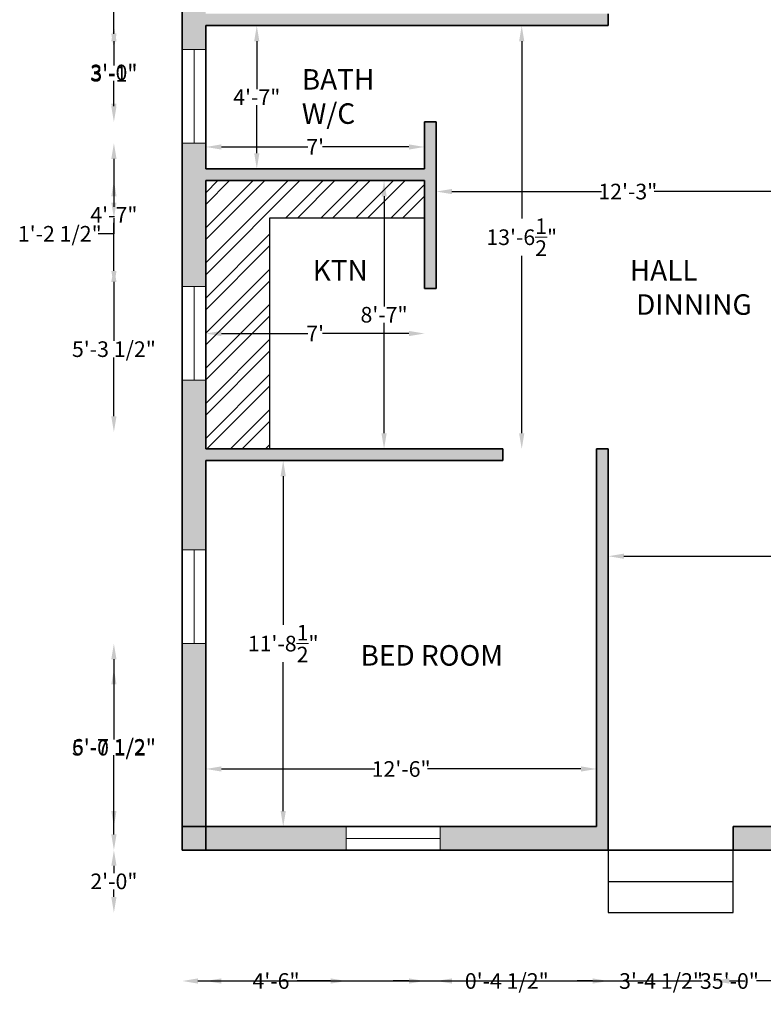
# Model space of a CAD drawing. Units: inches. Extents: x 759 to 1283, y 452 to 1038.
# Tile 1 of 3: x 759 to 1044, y 452 to 830. Entities that reach past the tile are written whole.
import ezdxf

# ---------------------------------------------------------------- set-up
doc = ezdxf.new("R2010")
doc.units = ezdxf.units.IN
for name, color, linetype, lineweight in [('A-AREA-IDEN', 1, 'Continuous', 25), ('A-COLS', 7, 'Continuous', 35), ('A-COLS-PATT', 7, 'Continuous', 13), ('A-FLOR-FIXT', 8, 'Continuous', 25), ('A-FLOR-FIXT-PATT', 7, 'Continuous', 13), ('DIM', 2, 'Continuous', 18), ('STAIR', 7, 'Continuous', 25), ('WALL', 7, 'Continuous', 35), ('WINDOWS', 4, 'Continuous', 18)]:
    doc.layers.add(name, color=color, linetype=linetype, lineweight=lineweight)
doc.layers.add('A-WALL-PATT', color=67, linetype='Continuous', lineweight=13, true_color=0x727430)
doc.styles.get("Standard").update_dxf_attribs({"font": 'arial.ttf'})
doc.dimstyles.get("Standard").update_dxf_attribs({"dimtxt": 6, "dimasz": 6, "dimexe": 0.18, "dimexo": 0.0625, "dimgap": 0.09, "dimtad": 0, "dimtih": 1, "dimtoh": 1, "dimdec": 4, "dimzin": 0, "dimdsep": 46, "dimlunit": 4, "dimtxsty": 'Standard', "dimcen": 0.09, "dimse1": 1, "dimse2": 1, "dimadec": 0, "dimazin": 0, "dimtfac": 1, "dimtdec": 4, "dimtofl": 0, "dimtmove": 0, "dimatfit": 3, "dimfxl": 1, "dimtolj": 1, "dimtzin": 0, "dimarcsym": 0})

# ---------------------------------------------------------------- blocks, each defined once
blk = doc.blocks.new('*D5')
at = {"layer": 'Defpoints', "color": 0, "transparency": 16777216}
for p in [(914.47, 780.7), (830.47, 772.31), (914.47, 772.31)]:
    blk.add_point(p, dxfattribs=at)
at = {"layer": 'DIM', "color": 0, "lineweight": -2, "transparency": 16777216}
for p, q in [((836.47, 780.7), (869.64, 780.7)), ((908.47, 780.7), (875.29, 780.7))]:
    blk.add_line(p, q, dxfattribs=at)
at = {"layer": 'DIM', "color": 0, "transparency": 16777216}
for points in [[(836.47, 781.7), (836.47, 779.7), (830.47, 780.7)], [(908.47, 781.7), (908.47, 779.7), (914.47, 780.7)]]:
    blk.add_solid(points, dxfattribs=at)
at = {"layer": 'DIM', "color": 0, "transparency": 16777216, "insert": (872.47, 780.7), "char_height": 6, "attachment_point": 5}
blk.add_mtext("\\A1;7'", dxfattribs=at)
blk = doc.blocks.new('*D6')
at = {"layer": 'Defpoints', "color": 0, "transparency": 16777216}
for p in [(830.47, 827.31), (830.47, 772.31), (850.06, 772.31)]:
    blk.add_point(p, dxfattribs=at)
at = {"layer": 'DIM', "color": 0, "lineweight": -2, "transparency": 16777216}
for p, q in [((850.06, 821.31), (850.06, 802.9)), ((850.06, 778.31), (850.06, 796.72))]:
    blk.add_line(p, q, dxfattribs=at)
at = {"layer": 'DIM', "color": 0, "transparency": 16777216}
for points in [[(849.06, 821.31), (851.06, 821.31), (850.06, 827.31)], [(849.06, 778.31), (851.06, 778.31), (850.06, 772.31)]]:
    blk.add_solid(points, dxfattribs=at)
at = {"layer": 'DIM', "color": 0, "transparency": 16777216, "insert": (850.06, 799.81), "char_height": 6, "attachment_point": 5}
blk.add_mtext('\\A1;4\'-7"', dxfattribs=at)
blk = doc.blocks.new('*D7')
at = {"layer": 'Defpoints', "color": 0, "transparency": 16777216}
for p in [(830.47, 767.81), (914.47, 767.81), (914.47, 709.09)]:
    blk.add_point(p, dxfattribs=at)
at = {"layer": 'DIM', "color": 0, "lineweight": -2, "transparency": 16777216}
for p, q in [((836.47, 709.09), (869.64, 709.09)), ((908.47, 709.09), (875.29, 709.09))]:
    blk.add_line(p, q, dxfattribs=at)
at = {"layer": 'DIM', "color": 0, "transparency": 16777216}
for points in [[(836.47, 710.09), (836.47, 708.09), (830.47, 709.09)], [(908.47, 710.09), (908.47, 708.09), (914.47, 709.09)]]:
    blk.add_solid(points, dxfattribs=at)
at = {"layer": 'DIM', "color": 0, "transparency": 16777216, "insert": (872.47, 709.09), "char_height": 6, "attachment_point": 5}
blk.add_mtext("\\A1;7'", dxfattribs=at)
blk = doc.blocks.new('*D8')
at = {"layer": 'Defpoints', "color": 0, "transparency": 16777216}
for p in [(830.47, 767.81), (830.47, 664.81), (898.91, 664.81)]:
    blk.add_point(p, dxfattribs=at)
at = {"layer": 'DIM', "color": 0, "lineweight": -2, "transparency": 16777216}
for p, q in [((898.91, 761.81), (898.91, 719.46)), ((898.91, 670.81), (898.91, 713.15))]:
    blk.add_line(p, q, dxfattribs=at)
at = {"layer": 'DIM', "color": 0, "transparency": 16777216}
for points in [[(897.91, 761.81), (899.91, 761.81), (898.91, 767.81)], [(897.91, 670.81), (899.91, 670.81), (898.91, 664.81)]]:
    blk.add_solid(points, dxfattribs=at)
at = {"layer": 'DIM', "color": 0, "transparency": 16777216, "insert": (898.91, 716.31), "char_height": 6, "attachment_point": 5}
blk.add_mtext('\\A1;8\'-7"', dxfattribs=at)
blk = doc.blocks.new('*D9')
at = {"layer": 'Defpoints', "color": 0, "transparency": 16777216}
for p in [(980.47, 541.94), (830.47, 519.81), (980.47, 519.81)]:
    blk.add_point(p, dxfattribs=at)
at = {"layer": 'DIM', "color": 0, "lineweight": -2, "transparency": 16777216}
for p, q in [((836.47, 541.94), (895.35, 541.94)), ((974.47, 541.94), (915.58, 541.94))]:
    blk.add_line(p, q, dxfattribs=at)
at = {"layer": 'DIM', "color": 0, "transparency": 16777216}
for points in [[(836.47, 542.94), (836.47, 540.94), (830.47, 541.94)], [(974.47, 542.94), (974.47, 540.94), (980.47, 541.94)]]:
    blk.add_solid(points, dxfattribs=at)
at = {"layer": 'DIM', "color": 0, "transparency": 16777216, "insert": (905.47, 541.94), "char_height": 6, "attachment_point": 5}
blk.add_mtext('\\A1;12\'-6"', dxfattribs=at)
blk = doc.blocks.new('*D10')
at = {"layer": 'Defpoints', "color": 0, "transparency": 16777216}
for p in [(830.47, 660.31), (830.47, 519.81), (860.2, 519.81)]:
    blk.add_point(p, dxfattribs=at)
at = {"layer": 'DIM', "color": 0, "lineweight": -2, "transparency": 16777216}
for p, q in [((860.2, 654.31), (860.2, 597.22)), ((860.2, 525.81), (860.2, 582.89))]:
    blk.add_line(p, q, dxfattribs=at)
at = {"layer": 'DIM', "color": 0, "transparency": 16777216}
for points in [[(859.2, 654.31), (861.2, 654.31), (860.2, 660.31)], [(859.2, 525.81), (861.2, 525.81), (860.2, 519.81)]]:
    blk.add_solid(points, dxfattribs=at)
at = {"layer": 'DIM', "color": 0, "transparency": 16777216, "insert": (860.2, 590.06), "char_height": 6, "attachment_point": 5}
blk.add_mtext('\\A1;11\'-8{\\H1x;\\S1/2;}"', dxfattribs=at)
blk = doc.blocks.new('*D12')
at = {"layer": 'Defpoints', "color": 0, "transparency": 16777216}
for p in [(1232.47, 623.61), (984.97, 524.08), (1232.47, 524.08)]:
    blk.add_point(p, dxfattribs=at)
at = {"layer": 'DIM', "color": 0, "lineweight": -2, "transparency": 16777216}
for p, q in [((990.97, 623.61), (1096.08, 623.61)), ((1226.47, 623.61), (1121.35, 623.61))]:
    blk.add_line(p, q, dxfattribs=at)
at = {"layer": 'DIM', "color": 0, "transparency": 16777216}
for points in [[(990.97, 624.61), (990.97, 622.61), (984.97, 623.61)], [(1226.47, 624.61), (1226.47, 622.61), (1232.47, 623.61)]]:
    blk.add_solid(points, dxfattribs=at)
at = {"layer": 'DIM', "color": 0, "transparency": 16777216, "insert": (1108.72, 623.61), "char_height": 6, "attachment_point": 5}
blk.add_mtext('\\A1;20\'-7{\\H1x;\\S1/2;}"', dxfattribs=at)
blk = doc.blocks.new('*D15')
at = {"layer": 'Defpoints', "color": 0, "transparency": 16777216}
for p in [(1065.97, 763.58), (918.97, 756.35), (1065.97, 756.35)]:
    blk.add_point(p, dxfattribs=at)
at = {"layer": 'DIM', "color": 0, "lineweight": -2, "transparency": 16777216}
for p, q in [((924.97, 763.58), (982.35, 763.58)), ((1059.97, 763.58), (1002.58, 763.58))]:
    blk.add_line(p, q, dxfattribs=at)
at = {"layer": 'DIM', "color": 0, "transparency": 16777216}
for points in [[(924.97, 764.58), (924.97, 762.58), (918.97, 763.58)], [(1059.97, 764.58), (1059.97, 762.58), (1065.97, 763.58)]]:
    blk.add_solid(points, dxfattribs=at)
at = {"layer": 'DIM', "color": 0, "transparency": 16777216, "insert": (992.47, 763.58), "char_height": 6, "attachment_point": 5}
blk.add_mtext('\\A1;12\'-3"', dxfattribs=at)
blk = doc.blocks.new('*D16')
at = {"layer": 'Defpoints', "color": 0, "transparency": 16777216}
for p in [(930.7, 827.31), (930.7, 664.81), (951.75, 664.81)]:
    blk.add_point(p, dxfattribs=at)
at = {"layer": 'DIM', "color": 0, "lineweight": -2, "transparency": 16777216}
for p, q in [((951.75, 821.31), (951.75, 753.22)), ((951.75, 670.81), (951.75, 738.89))]:
    blk.add_line(p, q, dxfattribs=at)
at = {"layer": 'DIM', "color": 0, "transparency": 16777216}
for points in [[(950.75, 821.31), (952.75, 821.31), (951.75, 827.31)], [(950.75, 670.81), (952.75, 670.81), (951.75, 664.81)]]:
    blk.add_solid(points, dxfattribs=at)
at = {"layer": 'DIM', "color": 0, "transparency": 16777216, "insert": (951.75, 746.06), "char_height": 6, "attachment_point": 5}
blk.add_mtext('\\A1;13\'-6{\\H1x;\\S1/2;}"', dxfattribs=at)
blk = doc.blocks.new('WIN-36IN')
for p, q in [((0, 0), (0, 9)), ((0, 9), (36, 9)), ((36, 9), (36, 0)), ((0, 4.5), (36, 4.5)), ((36, 0), (0, 0))]:
    blk.add_line(p, q)
blk = doc.blocks.new('COL-9X9IN')
for p, q in [((0, 0), (0, 9)), ((0, 9), (9, 9)), ((9, 9), (9, 0)), ((9, 0), (0, 0))]:
    blk.add_line(p, q)
blk = doc.blocks.new('*D23')
at = {"layer": 'Defpoints', "color": 0, "transparency": 16777216}
for p in [(821.47, 510.81), (1241.47, 510.81), (1241.47, 460.56)]:
    blk.add_point(p, dxfattribs=at)
at = {"layer": 'DIM', "color": 0, "lineweight": -2, "transparency": 16777216}
for p, q in [((827.47, 460.56), (1021.07, 460.56)), ((1235.47, 460.56), (1041.86, 460.56))]:
    blk.add_line(p, q, dxfattribs=at)
at = {"layer": 'DIM', "color": 0, "transparency": 16777216}
for points in [[(827.47, 461.56), (827.47, 459.56), (821.47, 460.56)], [(1235.47, 461.56), (1235.47, 459.56), (1241.47, 460.56)]]:
    blk.add_solid(points, dxfattribs=at)
at = {"layer": 'DIM', "color": 0, "transparency": 16777216, "insert": (1031.47, 460.56), "char_height": 6, "attachment_point": 5}
blk.add_mtext('\\A1;35\'-0"', dxfattribs=at)
blk = doc.blocks.new('*D24')
at = {"layer": 'Defpoints', "color": 0, "transparency": 16777216}
for p in [(1070.47, 1002.81), (1267.72, 1002.81), (1032.97, 486.81)]:
    blk.add_point(p, dxfattribs=at)
at = {"layer": 'DIM', "color": 0, "lineweight": -2, "transparency": 16777216}
for p, q in [((1267.72, 996.81), (1267.72, 747.96)), ((1267.72, 492.81), (1267.72, 741.65))]:
    blk.add_line(p, q, dxfattribs=at)
at = {"layer": 'DIM', "color": 0, "transparency": 16777216}
for points in [[(1266.72, 996.81), (1268.72, 996.81), (1267.72, 1002.81)], [(1266.72, 492.81), (1268.72, 492.81), (1267.72, 486.81)]]:
    blk.add_solid(points, dxfattribs=at)
at = {"layer": 'DIM', "color": 0, "transparency": 16777216, "insert": (1267.72, 744.81), "char_height": 6, "attachment_point": 5}
blk.add_mtext('\\A1;43\'-0"', dxfattribs=at)
blk = doc.blocks.new('*D27')
at = {"layer": 'Defpoints', "color": 0, "transparency": 16777216}
for p in [(1032.97, 1029.06), (984.97, 510.81), (1032.97, 510.81)]:
    blk.add_point(p, dxfattribs=at)
at = {"layer": 'DIM', "color": 0, "lineweight": -2, "transparency": 16777216}
for p, q in [((990.97, 1029.06), (1000.78, 1029.06)), ((1026.97, 1029.06), (1017.15, 1029.06))]:
    blk.add_line(p, q, dxfattribs=at)
at = {"layer": 'DIM', "color": 0, "transparency": 16777216}
for points in [[(990.97, 1030.06), (990.97, 1028.06), (984.97, 1029.06)], [(1026.97, 1030.06), (1026.97, 1028.06), (1032.97, 1029.06)]]:
    blk.add_solid(points, dxfattribs=at)
at = {"layer": 'DIM', "color": 0, "transparency": 16777216, "insert": (1008.97, 1029.06), "char_height": 6, "attachment_point": 5}
blk.add_mtext('\\A1;4\'-0"', dxfattribs=at)
blk = doc.blocks.new('*D28')
at = {"layer": 'Defpoints', "color": 0, "transparency": 16777216}
for p in [(795.22, 510.81), (984.97, 510.81), (984.97, 486.81)]:
    blk.add_point(p, dxfattribs=at)
at = {"layer": 'DIM', "color": 0, "lineweight": -2, "transparency": 16777216}
for p, q in [((795.22, 504.81), (795.22, 501.96)), ((795.22, 492.81), (795.22, 495.65))]:
    blk.add_line(p, q, dxfattribs=at)
at = {"layer": 'DIM', "color": 0, "transparency": 16777216}
for points in [[(794.22, 504.81), (796.22, 504.81), (795.22, 510.81)], [(794.22, 492.81), (796.22, 492.81), (795.22, 486.81)]]:
    blk.add_solid(points, dxfattribs=at)
at = {"layer": 'DIM', "color": 0, "transparency": 16777216, "insert": (795.22, 498.81), "char_height": 6, "attachment_point": 5}
blk.add_mtext('\\A1;2\'-0"', dxfattribs=at)
blk = doc.blocks.new('*D29')
at = {"layer": 'Defpoints', "color": 0, "transparency": 16777216}
for p in [(830.47, 981.81), (884.41, 981.81), (884.41, 460.56)]:
    blk.add_point(p, dxfattribs=at)
at = {"layer": 'DIM', "color": 0, "lineweight": -2, "transparency": 16777216}
for p, q in [((836.47, 460.56), (849.25, 460.56)), ((878.41, 460.56), (865.62, 460.56))]:
    blk.add_line(p, q, dxfattribs=at)
at = {"layer": 'DIM', "color": 0, "transparency": 16777216}
for points in [[(836.47, 461.56), (836.47, 459.56), (830.47, 460.56)], [(878.41, 461.56), (878.41, 459.56), (884.41, 460.56)]]:
    blk.add_solid(points, dxfattribs=at)
at = {"layer": 'DIM', "color": 0, "transparency": 16777216, "insert": (857.44, 460.56), "char_height": 6, "attachment_point": 5}
blk.add_mtext('\\A1;4\'-6"', dxfattribs=at)
blk = doc.blocks.new('*D31')
at = {"layer": 'Defpoints', "color": 0, "transparency": 16777216}
for p in [(884.41, 1029.06), (830.47, 519.81), (884.41, 519.81)]:
    blk.add_point(p, dxfattribs=at)
at = {"layer": 'DIM', "color": 0, "lineweight": -2, "transparency": 16777216}
for p, q in [((836.47, 1029.06), (849.25, 1029.06)), ((878.41, 1029.06), (865.62, 1029.06))]:
    blk.add_line(p, q, dxfattribs=at)
at = {"layer": 'DIM', "color": 0, "transparency": 16777216}
for points in [[(836.47, 1030.06), (836.47, 1028.06), (830.47, 1029.06)], [(878.41, 1030.06), (878.41, 1028.06), (884.41, 1029.06)]]:
    blk.add_solid(points, dxfattribs=at)
at = {"layer": 'DIM', "color": 0, "transparency": 16777216, "insert": (857.44, 1029.06), "char_height": 6, "attachment_point": 5}
blk.add_mtext('\\A1;4\'-6"', dxfattribs=at)
blk = doc.blocks.new('*D34')
at = {"layer": 'Defpoints', "color": 0, "transparency": 16777216}
for p in [(821.47, 906.81), (795.22, 818.14), (821.47, 818.14)]:
    blk.add_point(p, dxfattribs=at)
at = {"layer": 'DIM', "color": 0, "lineweight": -2, "transparency": 16777216}
for p, q in [((795.22, 900.81), (795.22, 865.67)), ((795.22, 824.14), (795.22, 859.28))]:
    blk.add_line(p, q, dxfattribs=at)
at = {"layer": 'DIM', "color": 0, "transparency": 16777216}
for points in [[(794.22, 900.81), (796.22, 900.81), (795.22, 906.81)], [(794.22, 824.14), (796.22, 824.14), (795.22, 818.14)]]:
    blk.add_solid(points, dxfattribs=at)
at = {"layer": 'DIM', "color": 0, "transparency": 16777216, "insert": (795.22, 862.47), "char_height": 6, "attachment_point": 5}
blk.add_mtext('\\A1;7\'-4 1/2"', dxfattribs=at)
blk = doc.blocks.new('*D35')
at = {"layer": 'Defpoints', "color": 0, "transparency": 16777216}
for p in [(821.47, 782.14), (795.22, 727.13), (821.47, 727.13)]:
    blk.add_point(p, dxfattribs=at)
at = {"layer": 'DIM', "color": 0, "lineweight": -2, "transparency": 16777216}
for p, q in [((795.22, 776.14), (795.22, 757.73)), ((795.22, 733.13), (795.22, 751.55))]:
    blk.add_line(p, q, dxfattribs=at)
at = {"layer": 'DIM', "color": 0, "transparency": 16777216}
for points in [[(794.22, 776.14), (796.22, 776.14), (795.22, 782.14)], [(794.22, 733.13), (796.22, 733.13), (795.22, 727.13)]]:
    blk.add_solid(points, dxfattribs=at)
at = {"layer": 'DIM', "color": 0, "transparency": 16777216, "insert": (795.22, 754.64), "char_height": 6, "attachment_point": 5}
blk.add_mtext('\\A1;4\'-7"', dxfattribs=at)
blk = doc.blocks.new('*D36')
at = {"layer": 'Defpoints', "color": 0, "transparency": 16777216}
for p in [(795.22, 590.06), (821.47, 590.06), (821.47, 510.81)]:
    blk.add_point(p, dxfattribs=at)
at = {"layer": 'DIM', "color": 0, "lineweight": -2, "transparency": 16777216}
for p, q in [((795.22, 584.06), (795.22, 553.62)), ((795.22, 516.81), (795.22, 547.24))]:
    blk.add_line(p, q, dxfattribs=at)
at = {"layer": 'DIM', "color": 0, "transparency": 16777216}
for points in [[(794.22, 584.06), (796.22, 584.06), (795.22, 590.06)], [(794.22, 516.81), (796.22, 516.81), (795.22, 510.81)]]:
    blk.add_solid(points, dxfattribs=at)
at = {"layer": 'DIM', "color": 0, "transparency": 16777216, "insert": (795.22, 550.43), "char_height": 6, "attachment_point": 5}
blk.add_mtext('\\A1;6\'-7 1/2"', dxfattribs=at)
blk = doc.blocks.new('*D38')
at = {"layer": 'Defpoints', "color": 0, "transparency": 16777216}
for p in [(795.22, 734.88), (1232.47, 734.88), (1232.47, 671.31)]:
    blk.add_point(p, dxfattribs=at)
at = {"layer": 'DIM', "color": 0, "lineweight": -2, "transparency": 16777216}
for p, q in [((795.22, 728.88), (795.22, 706.29)), ((795.22, 677.31), (795.22, 699.9))]:
    blk.add_line(p, q, dxfattribs=at)
at = {"layer": 'DIM', "color": 0, "transparency": 16777216}
for points in [[(794.22, 728.88), (796.22, 728.88), (795.22, 734.88)], [(794.22, 677.31), (796.22, 677.31), (795.22, 671.31)]]:
    blk.add_solid(points, dxfattribs=at)
at = {"layer": 'DIM', "color": 0, "transparency": 16777216, "insert": (795.22, 703.09), "char_height": 6, "attachment_point": 5}
blk.add_mtext('\\A1;5\'-3 1/2"', dxfattribs=at)
blk = doc.blocks.new('*D39')
at = {"layer": 'Defpoints', "color": 0, "transparency": 16777216}
for p in [(795.22, 580.37), (1232.47, 580.37), (1232.47, 519.81)]:
    blk.add_point(p, dxfattribs=at)
at = {"layer": 'DIM', "color": 0, "lineweight": -2, "transparency": 16777216}
for p, q in [((795.22, 574.37), (795.22, 553.28)), ((795.22, 525.81), (795.22, 546.89))]:
    blk.add_line(p, q, dxfattribs=at)
at = {"layer": 'DIM', "color": 0, "transparency": 16777216}
for points in [[(794.22, 574.37), (796.22, 574.37), (795.22, 580.37)], [(794.22, 525.81), (796.22, 525.81), (795.22, 519.81)]]:
    blk.add_solid(points, dxfattribs=at)
at = {"layer": 'DIM', "color": 0, "transparency": 16777216, "insert": (795.22, 550.09), "char_height": 6, "attachment_point": 5}
blk.add_mtext('\\A1;5\'-0 1/2"', dxfattribs=at)
blk = doc.blocks.new('*D41')
at = {"layer": 'Defpoints', "color": 0, "transparency": 16777216}
for p in [(984.966986, 872.954802), (1025.466986, 872.954802), (1025.466986, 460.55698)]:
    blk.add_point(p, dxfattribs=at)
at = {"layer": 'DIM', "color": 0, "lineweight": -2, "transparency": 16777216}
for p, q in [((978.966986, 460.55698), (972.966986, 460.55698)), ((1031.466986, 460.55698), (1037.466986, 460.55698))]:
    blk.add_line(p, q, dxfattribs=at)
at = {"layer": 'DIM', "color": 0, "transparency": 16777216}
for points in [[(978.966986, 461.55698), (978.966986, 459.55698), (984.966986, 460.55698)], [(1031.466986, 461.55698), (1031.466986, 459.55698), (1025.466986, 460.55698)]]:
    blk.add_solid(points, dxfattribs=at)
at = {"layer": 'DIM', "color": 0, "transparency": 16777216, "insert": (1005.216986, 460.55698), "char_height": 6, "attachment_point": 5}
blk.add_mtext('\\A1;3\'-4 1/2"', dxfattribs=at)
blk = doc.blocks.new('*D43')
at = {"layer": 'Defpoints', "color": 0, "transparency": 16777216}
for p in [(1070.47, 827.31), (795.22, 791.31), (1070.47, 791.31)]:
    blk.add_point(p, dxfattribs=at)
at = {"layer": 'DIM', "color": 0, "lineweight": -2, "transparency": 16777216}
for p, q in [((795.22, 821.31), (795.22, 812.46)), ((795.22, 797.31), (795.22, 806.15))]:
    blk.add_line(p, q, dxfattribs=at)
at = {"layer": 'DIM', "color": 0, "transparency": 16777216}
for points in [[(794.22, 821.31), (796.22, 821.31), (795.22, 827.31)], [(794.22, 797.31), (796.22, 797.31), (795.22, 791.31)]]:
    blk.add_solid(points, dxfattribs=at)
at = {"layer": 'DIM', "color": 0, "transparency": 16777216, "insert": (795.22, 809.31), "char_height": 6, "attachment_point": 5}
blk.add_mtext('\\A1;3\'-0"', dxfattribs=at)
blk = doc.blocks.new('*D44')
at = {"layer": 'Defpoints', "color": 0, "transparency": 16777216}
for p in [(795.22, 827.31), (984.97, 827.31), (914.47, 790.31)]:
    blk.add_point(p, dxfattribs=at)
at = {"layer": 'DIM', "color": 0, "lineweight": -2, "transparency": 16777216}
for p, q in [((795.22, 821.31), (795.22, 811.96)), ((795.22, 796.31), (795.22, 805.65))]:
    blk.add_line(p, q, dxfattribs=at)
at = {"layer": 'DIM', "color": 0, "transparency": 16777216}
for points in [[(794.22, 821.31), (796.22, 821.31), (795.22, 827.31)], [(794.22, 796.31), (796.22, 796.31), (795.22, 790.31)]]:
    blk.add_solid(points, dxfattribs=at)
at = {"layer": 'DIM', "color": 0, "transparency": 16777216, "insert": (795.22, 808.81), "char_height": 6, "attachment_point": 5}
blk.add_mtext('\\A1;3\'-1"', dxfattribs=at)
blk = doc.blocks.new('*D45')
at = {"layer": 'Defpoints', "color": 0, "transparency": 16777216}
for p in [(918.97, 726.32), (980.47, 664.81), (1267.72, 664.81)]:
    blk.add_point(p, dxfattribs=at)
at = {"layer": 'DIM', "color": 0, "lineweight": -2, "transparency": 16777216}
for p, q in [((1267.72, 720.32), (1267.72, 698.76)), ((1267.72, 670.81), (1267.72, 692.37))]:
    blk.add_line(p, q, dxfattribs=at)
at = {"layer": 'DIM', "color": 0, "transparency": 16777216}
for points in [[(1266.72, 720.32), (1268.72, 720.32), (1267.72, 726.32)], [(1266.72, 670.81), (1268.72, 670.81), (1267.72, 664.81)]]:
    blk.add_solid(points, dxfattribs=at)
at = {"layer": 'DIM', "color": 0, "transparency": 16777216, "insert": (1267.72, 695.57), "char_height": 6, "attachment_point": 5}
blk.add_mtext('\\A1;5\'-1 1/2"', dxfattribs=at)
blk = doc.blocks.new('*D46')
at = {"layer": 'Defpoints', "color": 0, "transparency": 16777216}
for p in [(980.47, 1029.06), (944.47, 660.31), (980.47, 660.31)]:
    blk.add_point(p, dxfattribs=at)
at = {"layer": 'DIM', "color": 0, "lineweight": -2, "transparency": 16777216}
for p, q in [((950.47, 1029.06), (954.4, 1029.06)), ((974.47, 1029.06), (970.53, 1029.06))]:
    blk.add_line(p, q, dxfattribs=at)
at = {"layer": 'DIM', "color": 0, "transparency": 16777216}
for points in [[(950.47, 1030.06), (950.47, 1028.06), (944.47, 1029.06)], [(974.47, 1030.06), (974.47, 1028.06), (980.47, 1029.06)]]:
    blk.add_solid(points, dxfattribs=at)
at = {"layer": 'DIM', "color": 0, "transparency": 16777216, "insert": (962.47, 1029.06), "char_height": 6, "attachment_point": 5}
blk.add_mtext('\\A1;3\'-0"', dxfattribs=at)
blk = doc.blocks.new('*D50')
at = {"layer": 'Defpoints', "color": 0, "transparency": 16777216}
for p in [(854.96, 1029.06), (830.47, 664.81), (854.96, 664.81)]:
    blk.add_point(p, dxfattribs=at)
at = {"layer": 'DIM', "color": 0, "lineweight": -2, "transparency": 16777216}
for p, q in [((836.47, 1029.06), (848.96, 1029.06)), ((854.96, 1029.06), (860.96, 1029.06))]:
    blk.add_line(p, q, dxfattribs=at)
at = {"layer": 'DIM', "color": 0, "transparency": 16777216}
for points in [[(836.47, 1030.06), (836.47, 1028.06), (830.47, 1029.06)], [(848.96, 1030.06), (848.96, 1028.06), (854.96, 1029.06)]]:
    blk.add_solid(points, dxfattribs=at)
at = {"layer": 'DIM', "color": 0, "transparency": 16777216, "insert": (876.07, 1029.06), "char_height": 6, "attachment_point": 5}
blk.add_mtext('\\A1;2\'-0 1/2"', dxfattribs=at)
blk = doc.blocks.new('*D51')
at = {"layer": 'Defpoints', "color": 0, "transparency": 16777216}
for p in [(914.47, 767.81), (795.22, 753.37), (914.47, 753.37)]:
    blk.add_point(p, dxfattribs=at)
at = {"layer": 'DIM', "color": 0, "lineweight": -2, "transparency": 16777216}
for p, q in [((795.22, 761.81), (795.22, 759.37)), ((795.22, 753.37), (795.22, 747.37)), ((795.22, 747.37), (789.22, 747.37))]:
    blk.add_line(p, q, dxfattribs=at)
at = {"layer": 'DIM', "color": 0, "transparency": 16777216}
for points in [[(794.22, 761.81), (796.22, 761.81), (795.22, 767.81)], [(794.22, 759.37), (796.22, 759.37), (795.22, 753.37)]]:
    blk.add_solid(points, dxfattribs=at)
at = {"layer": 'DIM', "color": 0, "transparency": 16777216, "insert": (774.44, 747.37), "char_height": 6, "attachment_point": 5}
blk.add_mtext('\\A1;1\'-2 1/2"', dxfattribs=at)
blk = doc.blocks.new('*D52')
at = {"layer": 'Defpoints', "color": 0, "transparency": 16777216}
for p in [(914.47, 726.32), (918.97, 726.32), (918.97, 460.56)]:
    blk.add_point(p, dxfattribs=at)
at = {"layer": 'DIM', "color": 0, "lineweight": -2, "transparency": 16777216}
for p, q in [((908.47, 460.56), (902.47, 460.56)), ((924.97, 460.56), (930.97, 460.56))]:
    blk.add_line(p, q, dxfattribs=at)
at = {"layer": 'DIM', "color": 0, "transparency": 16777216}
for points in [[(908.47, 461.56), (908.47, 459.56), (914.47, 460.56)], [(924.97, 461.56), (924.97, 459.56), (918.97, 460.56)]]:
    blk.add_solid(points, dxfattribs=at)
at = {"layer": 'DIM', "color": 0, "transparency": 16777216, "insert": (946.02, 460.56), "char_height": 6, "attachment_point": 5}
blk.add_mtext('\\A1;0\'-4 1/2"', dxfattribs=at)

msp = doc.modelspace()

# ---------------------------------------------------------------- hatches: boundary and pattern name
at = {"layer": 'A-COLS-PATT'}
h = msp.add_hatch(color=256, dxfattribs=at)
h.dxf.hatch_style = 1
h.paths.add_polyline_path([(1241.46699, 990.80698), (1232.46699, 990.80698), (1232.46699, 981.80698), (1241.46699, 981.80698)])
h.paths.add_polyline_path([(830.46699, 990.80698), (821.46699, 990.80698), (821.46699, 981.80698), (830.46699, 981.80698)])
h.paths.add_polyline_path([(830.46699, 519.80698), (821.46699, 519.80698), (821.46699, 510.80698), (830.46699, 510.80698)])
h.paths.add_polyline_path([(1241.46699, 519.80698), (1232.46699, 519.80698), (1232.46699, 510.80698), (1241.46699, 510.80698)])
at = {"layer": 'A-FLOR-FIXT-PATT'}
h = msp.add_hatch(dxfattribs=at)
h.set_pattern_fill('ANSI32', color=256)
h.paths.add_polyline_path([(854.96067, 753.37274), (914.46699, 753.37274), (914.46699, 767.80698), (830.46699, 767.80698), (830.46699, 664.80698), (854.96067, 664.80698)])
at = {"layer": 'A-WALL-PATT'}
h = msp.add_hatch(color=256, dxfattribs=at)
h.dxf.hatch_style = 1
h.paths.add_polyline_path([(1232.46699, 519.80698), (1159.97269, 519.80698), (1159.97269, 510.80698), (1232.46699, 510.80698)])
h.paths.add_polyline_path([(1241.46699, 580.365), (1232.46699, 580.365), (1232.46699, 519.80698), (1241.46699, 519.80698)])
h.paths.add_polyline_path([(1123.97269, 519.80698), (1032.96699, 519.80698), (1032.96699, 510.80698), (1123.97269, 510.80698)])
h.paths.add_polyline_path([(984.96699, 519.80698), (984.96699, 664.80698), (980.46699, 664.80698), (980.46699, 660.30698), (980.46699, 519.80698), (920.40841, 519.80698), (920.40841, 510.80698), (984.96699, 510.80698)])
h.paths.add_polyline_path([(884.40841, 519.80698), (830.46699, 519.80698), (830.46699, 510.80698), (884.40841, 510.80698)])
h.paths.add_polyline_path([(830.46699, 590.05698), (821.46699, 590.05698), (821.46699, 519.80698), (830.46699, 519.80698)])
h.paths.add_polyline_path([(830.46699, 660.30698), (944.46699, 660.30698), (944.46699, 664.80698), (830.46699, 664.80698), (830.46699, 691.13164), (821.46699, 691.13164), (821.46699, 626.05698), (830.46699, 626.05698)])
h.paths.add_polyline_path([(830.46699, 767.80698), (914.46699, 767.80698), (914.46699, 726.32345), (918.96699, 726.32345), (918.96699, 775.80521), (918.96699, 790.30698), (914.46699, 790.30698), (914.46699, 772.30698), (830.46699, 772.30698), (830.46699, 782.14186), (821.46699, 782.14186), (821.46699, 727.13164), (830.46699, 727.13164)])
h.paths.add_polyline_path([(830.46699, 906.80698), (821.46699, 906.80698), (821.46699, 818.14186), (830.46699, 818.14186), (830.46699, 827.30698), (984.96699, 827.30698), (984.96699, 831.80698), (980.46699, 831.80698), (830.46699, 831.80698)])
h.paths.add_polyline_path([(830.46699, 981.80698), (821.46699, 981.80698), (821.46699, 942.80698), (830.46699, 942.80698)])
h.paths.add_polyline_path([(884.40841, 990.80698), (830.46699, 990.80698), (830.46699, 981.80698), (884.40841, 981.80698)])
h.paths.add_polyline_path([(984.96699, 998.30698), (1065.96699, 998.30698), (1065.96699, 981.80698), (1065.96699, 867.80698), (1070.46699, 867.80698), (1070.46699, 981.80698), (1139.68016, 981.80698), (1139.68016, 990.80698), (1070.46699, 990.80698), (1070.46699, 1002.80698), (980.46699, 1002.80698), (980.46699, 990.80698), (920.40841, 990.80698), (920.40841, 981.80698), (980.46699, 981.80698), (980.46699, 867.80698), (984.96699, 867.80698), (984.96699, 981.80698)])
h.paths.add_polyline_path([(1232.46699, 990.80698), (1175.68016, 990.80698), (1175.68016, 981.80698), (1232.46699, 981.80698)])
h.paths.add_polyline_path([(1241.46699, 981.80698), (1232.46699, 981.80698), (1232.46699, 947.03418), (1241.46699, 947.03418)])
h.paths.add_polyline_path([(1241.46699, 911.03418), (1232.46699, 911.03418), (1232.46699, 831.80698), (1070.46699, 831.80698), (1065.96699, 831.80698), (1065.96699, 827.30698), (1070.46699, 827.30698), (1232.46699, 827.30698), (1232.46699, 770.87725), (1241.46699, 770.87725)])
h.paths.add_polyline_path([(1241.46699, 734.87725), (1232.46699, 734.87725), (1232.46699, 671.30698), (1070.46699, 671.30698), (1070.46699, 666.80698), (1232.46699, 666.80698), (1232.46699, 616.365), (1241.46699, 616.365)])
h.paths.add_polyline_path([(1070.46699, 791.30698), (1065.96699, 791.30698), (1065.96699, 666.80698), (1070.46699, 666.80698)])

# ---------------------------------------------------------------- linework, layer by layer
at = {"layer": 'A-FLOR-FIXT'}
for p, q in [((914.46699, 753.37274), (854.96067, 753.37274)), ((854.96067, 753.37274), (854.96067, 664.80698))]:
    msp.add_line(p, q, dxfattribs=at)
at = {"layer": 'STAIR'}
for p, q in [((984.96699, 510.80698), (984.96699, 486.80698)), ((1032.96699, 486.80698), (1032.96699, 510.80698)), ((984.96699, 498.80698), (1020.96699, 498.80698)), ((1020.96699, 498.80698), (1032.96699, 498.80698)), ((984.96699, 486.80698), (1020.96699, 486.80698)), ((1020.96699, 486.80698), (1032.96699, 486.80698))]:
    msp.add_line(p, q, dxfattribs=at)
at = {"layer": 'WALL'}
for p, q in [((821.46699, 990.80698), (821.46699, 510.80698)), ((984.96699, 831.80698), (984.96699, 827.30698)), ((830.46699, 827.30698), (984.96699, 827.30698)), ((830.46699, 827.30698), (830.46699, 772.30698)), ((914.46699, 790.30698), (914.46699, 772.30698)), ((914.46699, 772.30698), (914.46699, 790.30698)), ((914.46699, 790.30698), (918.96699, 790.30698)), ((918.96699, 790.30698), (918.96699, 772.30698)), ((918.96699, 790.30698), (918.96699, 772.30698)), ((918.96699, 775.80521), (918.96699, 726.32345)), ((830.46699, 772.30698), (914.46699, 772.30698)), ((830.46699, 767.80698), (914.46699, 767.80698)), ((830.46699, 767.80698), (830.46699, 664.80698)), ((914.46699, 726.32345), (914.46699, 767.80698)), ((918.96699, 726.32345), (914.46699, 726.32345)), ((830.46699, 664.80698), (944.46699, 664.80698)), ((944.46699, 660.30698), (944.46699, 664.80698)), ((980.46699, 660.30698), (980.46699, 664.80698)), ((980.46699, 664.80698), (984.96699, 664.80698)), ((984.96699, 664.80698), (984.96699, 519.80698)), ((830.46699, 660.30698), (944.46699, 660.30698)), ((830.46699, 660.30698), (830.46699, 519.80698)), ((980.46699, 660.30698), (980.46699, 519.80698)), ((830.46699, 519.80698), (980.46699, 519.80698)), ((984.96699, 519.80698), (984.96699, 510.80698)), ((1032.96699, 519.80698), (1232.46699, 519.80698)), ((1032.96699, 510.80698), (1032.96699, 519.80698)), ((821.46699, 510.80698), (1241.46699, 510.80698))]:
    msp.add_line(p, q, dxfattribs=at)

# ---------------------------------------------------------------- block references
at = {"layer": 'A-COLS', "rotation": 180}
msp.add_blockref('COL-9X9IN', (830.46697, 519.80696), dxfattribs=at)
at = {"layer": 'WINDOWS'}
for p, rotation in [((821.46701, 818.14227), 270.0000000000004), ((821.46701, 727.13205), 270.0000000000001), ((821.46701, 626.05739), 270.0000000000001)]:
    msp.add_blockref('WIN-36IN', p, dxfattribs=dict(at, rotation=rotation))
msp.add_blockref('WIN-36IN', (884.408, 510.807), dxfattribs=at)

# ---------------------------------------------------------------- texts
at = {"layer": 'A-AREA-IDEN', "char_height": 7.875, "attachment_point": 1}
for s, insert in [('BATH \\PW/C', (867.32718, 810.57964)), ('KTN', (871.51154, 737.27594)), ('HALL\\P DINNING', (993.23019, 737.27594)), ('BED ROOM', (889.88863, 589.48127))]:
    msp.add_mtext_dynamic_manual_height_columns(s, width=120.4934303, gutter_width=39.375, heights=[0], dxfattribs=dict(at, insert=insert))

# ---------------------------------------------------------------- dimensions: what is measured, and where the dimension line sits
at = {"layer": 'DIM'}
for base, p1, p2, override, picture, middle in [((854.96067, 1029.05698), (830.46699, 664.80698), (854.96067, 664.80698), {"dimdec": 1, "dimlfac": 1, "dimrnd": 0, "dimzin": 1, "dimdsep": 46, "dimlunit": 4, "dimfrac": 2}, '*D50', (876.06704, 1029.05698)), ((884.40841, 1029.05698), (830.46699, 519.80698), (884.40841, 519.80698), {"dimdec": 1, "dimlfac": 1, "dimrnd": 0, "dimzin": 1, "dimdsep": 46, "dimlunit": 4, "dimfrac": 2}, '*D31', (857.4377, 1029.05698)), ((980.46699, 1029.05698), (944.46699, 660.30698), (980.46699, 660.30698), {"dimdec": 1, "dimlfac": 1, "dimrnd": 0, "dimzin": 1, "dimdsep": 46, "dimlunit": 4, "dimfrac": 2}, '*D46', (962.46699, 1029.05698)), ((1032.96699, 1029.05698), (984.96699, 510.80698), (1032.96699, 510.80698), {"dimdec": 1, "dimlfac": 1, "dimrnd": 0, "dimzin": 1, "dimdsep": 46, "dimlunit": 4, "dimfrac": 2}, '*D27', (1008.96699, 1029.05698)), ((884.40841, 460.55698), (830.46699, 981.80698), (884.40841, 981.80698), {"dimdec": 1, "dimlfac": 1, "dimrnd": 0, "dimzin": 1, "dimdsep": 46, "dimlunit": 4, "dimfrac": 2}, '*D29', (857.4377, 460.55698)), ((1025.46699, 460.55698), (984.96699, 872.9548), (1025.46699, 872.9548), {"dimdec": 1, "dimlfac": 1, "dimrnd": 0, "dimzin": 1, "dimdsep": 46, "dimlunit": 4, "dimfrac": 2}, '*D41', (1005.21699, 460.55698)), ((914.46699, 780.69553), (830.46699, 772.30698), (914.46699, 772.30698), {"dimclrd": 0, "dimclre": 0, "dimclrt": 0}, '*D5', (872.46699, 780.69553)), ((914.46699, 709.08986), (830.46699, 767.80698), (914.46699, 767.80698), {"dimclrd": 0, "dimclre": 0, "dimclrt": 0}, '*D7', (872.46699, 709.08986)), ((1065.96699, 763.57787), (918.96699, 756.34782), (1065.96699, 756.34782), {"dimclrd": 0, "dimclre": 0, "dimclrt": 0}, '*D15', (992.46699, 763.57787)), ((918.96699, 460.55698), (914.46699, 726.32345), (918.96699, 726.32345), {"dimdec": 1, "dimlfac": 1, "dimrnd": 0, "dimzin": 1, "dimdsep": 46, "dimlunit": 4, "dimfrac": 2}, '*D52', (946.0222, 460.55698)), ((1232.46699, 623.61456), (984.96699, 524.07962), (1232.46699, 524.07962), {"dimclrd": 0, "dimclre": 0, "dimclrt": 0}, '*D12', (1108.71699, 623.61456)), ((980.46699, 541.93548), (830.46699, 519.80698), (980.46699, 519.80698), {"dimclrd": 0, "dimclre": 0, "dimclrt": 0}, '*D9', (905.46699, 541.93548)), ((1241.46699, 460.55698), (821.46699, 510.80698), (1241.46699, 510.80698), {"dimdec": 1, "dimlfac": 1, "dimrnd": 0, "dimzin": 1, "dimdsep": 46, "dimlunit": 4, "dimfrac": 2}, '*D23', (1031.46699, 460.55698))]:
    dim = msp.add_linear_dim(base=base, p1=p1, p2=p2, dimstyle='Standard', override=override, dxfattribs=at)
    dim.commit()
    dim.dimension.update_dxf_attribs({"geometry": picture, "text_midpoint": middle})
for base, p1, p2, override, picture, middle in [((1267.71699, 1002.80698), (1032.96699, 486.80698), (1070.46699, 1002.80698), {"dimdec": 1, "dimlfac": 1, "dimrnd": 0, "dimzin": 1, "dimdsep": 46, "dimlunit": 4, "dimfrac": 2}, '*D24', (1267.71699, 744.80698)), ((795.21699, 818.14186), (821.46699, 906.80698), (821.46699, 818.14186), {"dimdec": 1, "dimlfac": 1, "dimrnd": 0, "dimzin": 1, "dimdsep": 46, "dimlunit": 4, "dimfrac": 2}, '*D34', (795.21699, 862.47442)), ((795.21699, 791.30698), (1070.46699, 827.30698), (1070.46699, 791.30698), {"dimdec": 1, "dimlfac": 1, "dimrnd": 0, "dimzin": 1, "dimdsep": 46, "dimlunit": 4, "dimfrac": 2}, '*D43', (795.21699, 809.30698)), ((795.21699, 827.30698), (914.46699, 790.30698), (984.96699, 827.30698), {"dimdec": 1, "dimlfac": 1, "dimrnd": 0, "dimzin": 1, "dimdsep": 46, "dimlunit": 4, "dimfrac": 2}, '*D44', (795.21699, 808.80698)), ((850.06218, 772.30698), (830.46699, 827.30698), (830.46699, 772.30698), {"dimclrd": 0, "dimclre": 0, "dimclrt": 0}, '*D6', (850.06218, 799.80698)), ((951.74978, 664.80698), (930.70435, 827.30698), (930.70435, 664.80698), {"dimclrd": 0, "dimclre": 0, "dimclrt": 0}, '*D16', (951.74978, 746.05698)), ((795.21699, 727.13164), (821.46699, 782.14186), (821.46699, 727.13164), {"dimdec": 1, "dimlfac": 1, "dimrnd": 0, "dimzin": 1, "dimdsep": 46, "dimlunit": 4, "dimfrac": 2}, '*D35', (795.21699, 754.63675)), ((795.21699, 753.37274), (914.46699, 767.80698), (914.46699, 753.37274), {"dimdec": 1, "dimlfac": 1, "dimrnd": 0, "dimzin": 1, "dimdsep": 46, "dimlunit": 4, "dimfrac": 2}, '*D51', (774.44418, 747.37274)), ((898.91146, 664.80698), (830.46699, 767.80698), (830.46699, 664.80698), {"dimclrd": 0, "dimclre": 0, "dimclrt": 0}, '*D8', (898.91146, 716.30698)), ((795.21699, 734.87725), (1232.46699, 671.30698), (1232.46699, 734.87725), {"dimdec": 1, "dimlfac": 1, "dimrnd": 0, "dimzin": 1, "dimdsep": 46, "dimlunit": 4, "dimfrac": 2}, '*D38', (795.21699, 703.09212)), ((1267.71699, 664.80698), (918.96699, 726.32345), (980.46699, 664.80698), {"dimdec": 1, "dimlfac": 1, "dimrnd": 0, "dimzin": 1, "dimdsep": 46, "dimlunit": 4, "dimfrac": 2}, '*D45', (1267.71699, 695.56521)), ((860.20108, 519.80698), (830.46699, 660.30698), (830.46699, 519.80698), {"dimclrd": 0, "dimclre": 0, "dimclrt": 0}, '*D10', (860.20108, 590.05698)), ((795.216986, 590.05698), (821.466986, 510.80698), (821.466986, 590.05698), {"dimdec": 1, "dimlfac": 1, "dimrnd": 0, "dimzin": 1, "dimdsep": 46, "dimlunit": 4, "dimfrac": 2}, '*D36', (795.216986, 550.43198)), ((795.21699, 580.365), (1232.46699, 519.80698), (1232.46699, 580.365), {"dimdec": 1, "dimlfac": 1, "dimrnd": 0, "dimzin": 1, "dimdsep": 46, "dimlunit": 4, "dimfrac": 2}, '*D39', (795.21699, 550.08599)), ((795.21699, 510.80698), (984.96699, 486.80698), (984.96699, 510.80698), {"dimdec": 1, "dimlfac": 1, "dimrnd": 0, "dimzin": 1, "dimdsep": 46, "dimlunit": 4, "dimfrac": 2}, '*D28', (795.21699, 498.80698))]:
    dim = msp.add_linear_dim(base=base, p1=p1, p2=p2, angle=90, dimstyle='Standard', override=override, dxfattribs=at)
    dim.commit()
    dim.dimension.update_dxf_attribs({"geometry": picture, "text_midpoint": middle})

doc.saveas('drawing.dxf')
